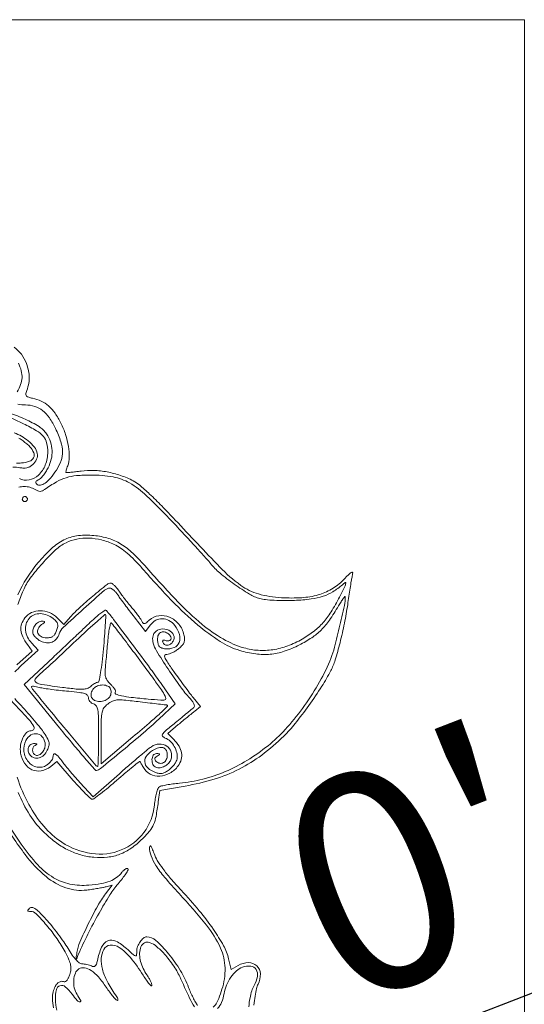
# Model space of a CAD drawing. Units: inches. Extents: x 2656 to 9931, y 1941 to 3068.
# Tile 41 of 46: x 2854 to 2868, y 2967 to 2994. Entities that reach past the tile are written whole.
import ezdxf

# ---------------------------------------------------------------- set-up
doc = ezdxf.new("R2010")
doc.units = ezdxf.units.IN
for name, color, linetype, lineweight in [('A-ANNO-DIMS', 2, 'Continuous', 18), ('A-ELEV-FNSH', 8, 'Continuous', 13), ('A-ELEV-ORN', 8, 'Continuous', 13)]:
    doc.layers.add(name, color=color, linetype=linetype, lineweight=lineweight)
doc.styles.get("Standard").update_dxf_attribs({"font": 'arial.ttf'})
doc.dimstyles.new('ISO-25', dxfattribs={"dimtxt": 6, "dimasz": 2.5, "dimexe": 1.25, "dimexo": 0.625, "dimtad": 1, "dimdec": 0, "dimlunit": 3, "dimtxsty": 'Standard', "dimcen": 2.5, "dimadec": 0, "dimazin": 0, "dimtfac": 1, "dimtdec": 0, "dimtmove": 0, "dimatfit": 3, "dimfxl": 1, "dimarcsym": 0})

# ---------------------------------------------------------------- blocks, each defined once
blk = doc.blocks.new('*D166')
at = {"layer": 'A-ANNO-DIMS', "color": 0, "lineweight": -2, "transparency": 16777216}
for p, q in [((2884.455, 2990.075), (2890.436, 2974.616)), ((2876.883, 2987.145), (2882.863, 2971.687)), ((2887.653, 2974.88), (2884.744, 2973.755)), ((2882.412, 2972.852), (2864.04, 2965.744))]:
    blk.add_line(p, q, dxfattribs=at)
at = {"layer": 'A-ANNO-DIMS', "color": 0, "transparency": 16777216}
for points in [[(2887.503, 2975.269), (2887.803, 2974.491), (2889.985, 2975.782)], [(2884.594, 2974.143), (2884.894, 2973.366), (2882.412, 2972.852)]]:
    blk.add_solid(points, dxfattribs=at)
at = {"layer": 'Defpoints', "color": 0, "transparency": 16777216}
for p in [(2884.229, 2990.658), (2876.657, 2987.728), (2882.412, 2972.852)]:
    blk.add_point(p, dxfattribs=at)
at = {"layer": 'A-ANNO-DIMS', "color": 0, "transparency": 16777216, "insert": (2870.73, 2972.287), "char_height": 6, "attachment_point": 5, "rotation": 21.1508}
blk.add_mtext('0\'-8"', dxfattribs=at)

msp = doc.modelspace()

# ---------------------------------------------------------------- linework, layer by layer
at = {"layer": 'A-ELEV-FNSH'}
msp.add_lwpolyline([(2826.64, 2994.347), (2868.226, 2994.347), (2868.226, 2892.035), (2826.64, 2892.035)], close=True, dxfattribs=at)
at = {"layer": 'A-ELEV-ORN'}
for points in [[(2854.23, 2972.992, 0.048806), (2854.547, 2972.366, 0.063105), (2854.957, 2971.872, 0.02947), (2855.295, 2971.591, 0.044031), (2855.623, 2971.392, 0.047712), (2855.96, 2971.264, 0.044288), (2856.323, 2971.198, 0.049374), (2856.702, 2971.201, 0.064618), (2857.039, 2971.282, 0.0621), (2857.354, 2971.45, 0.04132), (2857.668, 2971.712, 0.02581), (2857.866, 2971.929, 0.071696), (2857.973, 2972.105, 0.05657), (2858.04, 2972.327, 0.011722), (2858.102, 2972.73), (2858.144, 2973.048), (2858.842, 2973.168, 0.031548), (2859.647, 2973.358, 0.043232), (2860.338, 2973.635, 0.043767), (2860.964, 2974.024, 0.033519), (2861.576, 2974.549, 0.030431), (2861.884, 2974.892, 0.012266), (2862.265, 2975.395, 0.012368), (2862.625, 2975.924, 0.025654), (2862.874, 2976.357, 0.043147), (2862.994, 2976.651, 0.012156), (2863.128, 2977.129, 0.012381), (2863.251, 2977.667, 0.014486), (2863.341, 2978.184, -0.001676), (2863.374, 2978.412, -0.001753), (2863.409, 2978.637, -0.001681), (2863.44, 2978.83, -0.007763), (2863.46, 2978.942, 0.019715), (2863.479, 2979.064, 0.552387), (2863.458, 2979.081, 0.111126), (2863.41, 2979.051, 0.002476), (2863.214, 2978.857, -0.063383), (2862.893, 2978.609, -0.063935), (2862.522, 2978.45, -0.054142), (2862.07, 2978.373, -0.029361), (2861.506, 2978.372, -0.053891), (2860.87, 2978.477, -0.09017), (2860.384, 2978.713, -0.042819), (2859.805, 2979.219, -0.004549), (2858.572, 2980.52, 0.007082), (2858.2, 2980.909, 0.010597), (2857.862, 2981.237, 0.010585), (2857.58, 2981.49, 0.059203), (2857.412, 2981.603, 0.036247), (2857.06, 2981.751, 0.035563), (2856.689, 2981.848, 0.036527), (2856.318, 2981.89, 0.044145), (2855.968, 2981.872, -0.004618), (2855.815, 2981.852, -0.007219), (2855.683, 2981.839, -0.002709), (2855.57, 2981.829, -0.203128), (2855.553, 2981.835, -0.261874), (2855.548, 2981.849, -0.014563), (2855.558, 2981.896, -0.019407), (2855.574, 2981.954, -0.012699), (2855.597, 2982.02, 0.08819), (2855.641, 2982.25, 0.042084), (2855.618, 2982.552, 0.038933), (2855.539, 2982.881, 0.03792), (2855.41, 2983.197, 0.036437), (2855.247, 2983.471, 0.060016), (2855.067, 2983.671, 0.06765), (2854.863, 2983.806, 0.063263), (2854.625, 2983.886, -0.025868), (2854.519, 2983.913, -0.107249), (2854.462, 2983.945, -0.189099), (2854.44, 2983.988, -0.116621), (2854.448, 2984.044, 0.038233), (2854.511, 2984.253, 0.051641), (2854.534, 2984.449, 0.05259), (2854.515, 2984.642, 0.041783), (2854.456, 2984.844, 0.070095), (2854.315, 2985.099, 0.078135), (2854.113, 2985.294, 0.079077)], [(2854.233, 2984.857, -0.044451), (2854.313, 2984.64, -0.078218), (2854.334, 2984.45, -0.079048), (2854.296, 2984.264, -0.046304), (2854.196, 2984.059, 0.047957)], [(2854.218, 2983.718, 0.03751), (2854.433, 2983.701, -0.076239), (2854.688, 2983.661, -0.090313), (2854.903, 2983.546, -0.076144), (2855.09, 2983.345, -0.038724), (2855.261, 2983.045, -0.028856), (2855.408, 2982.681, -0.076946), (2855.456, 2982.407, -0.092728), (2855.415, 2982.161, -0.056238), (2855.283, 2981.897, -0.029077), (2855.122, 2981.678, -0.064736), (2854.971, 2981.537, -0.108333), (2854.842, 2981.481, -0.248543), (2854.744, 2981.512, -0.080101), (2854.718, 2981.548, -0.211882), (2854.716, 2981.579, -0.164265), (2854.739, 2981.606, -0.045944), (2854.79, 2981.631, 0.10487), (2854.846, 2981.668, 0.027488), (2854.918, 2981.748, 0.026679), (2854.991, 2981.85, 0.024525), (2855.055, 2981.962, 0.060506), (2855.142, 2982.199, 0.069274), (2855.164, 2982.44, 0.069972), (2855.12, 2982.676, 0.063577), (2855.012, 2982.898, 0.107608), (2854.805, 2983.101, 0.034268), (2854.424, 2983.306, 0.034451), (2853.986, 2983.469, 0.051823)], [(2853.842, 2983.44), (2854.371, 2983.182, -0.01869), (2854.737, 2982.986, -0.082984), (2854.924, 2982.831, -0.119266), (2855.015, 2982.653, -0.059157), (2855.045, 2982.4, -0.092228), (2854.978, 2982.042, -0.113061), (2854.789, 2981.761, -0.138967), (2854.528, 2981.626, -0.173005), (2854.26, 2981.665, -0.048254)], [(2854.084, 2981.976, -0.070536), (2854.276, 2981.965, 0.042314), (2854.38, 2981.954, 0.065901), (2854.469, 2981.963, 0.070033), (2854.549, 2981.994, 0.055283), (2854.625, 2982.049, 0.102685), (2854.735, 2982.2, 0.153719), (2854.755, 2982.361, 0.121971), (2854.677, 2982.531, 0.052991), (2854.502, 2982.71, 0.090302), (2854.115, 2982.926, 0.071489)], [(2854.25, 2982.779, -0.019972), (2854.361, 2982.707, -0.019921), (2854.467, 2982.624, -0.031903), (2854.55, 2982.545, -0.083683), (2854.659, 2982.379, -0.226186), (2854.654, 2982.241, -0.19243), (2854.54, 2982.143, -0.0618), (2854.317, 2982.096, -0.017844), (2854.177, 2982.089, -0.111032)], [(2854.248, 2981.426, -0.071275), (2854.394, 2981.446, -0.065833), (2854.553, 2981.424, -0.072585), (2854.695, 2981.362, 0.038782), (2854.771, 2981.322, 0.100434), (2854.831, 2981.31, 0.107028), (2854.889, 2981.322, 0.047721), (2854.957, 2981.361, -0.022709), (2855.289, 2981.574, -0.055018), (2855.556, 2981.69, -0.05461), (2855.842, 2981.747, -0.022094), (2856.241, 2981.763, -0.042989), (2856.854, 2981.709, -0.087275), (2857.308, 2981.544, -0.060467), (2857.777, 2981.192, -0.012478), (2858.505, 2980.458, -0.001643), (2858.857, 2980.083, -0.002101), (2859.179, 2979.734, -0.001624), (2859.446, 2979.44, -0.017799), (2859.549, 2979.318, 0.052744), (2859.8, 2979.059, 0.019241), (2860.205, 2978.746, 0.018442), (2860.624, 2978.47, 0.070736), (2860.911, 2978.347, 0.041481), (2861.066, 2978.319, 0.011613), (2861.311, 2978.301, 0.01162), (2861.59, 2978.293, 0.011922), (2861.867, 2978.298, 0.019879), (2862.329, 2978.337, 0.048301), (2862.662, 2978.411, 0.059001), (2862.933, 2978.537, 0.045481), (2863.194, 2978.732, -0.048141), (2863.271, 2978.789, -0.666317), (2863.291, 2978.774, -0.055029), (2863.257, 2978.682, -0.002672), (2863.111, 2978.39, -0.020952), (2862.881, 2977.98, -0.042924), (2862.661, 2977.684, -0.047406), (2862.409, 2977.449, -0.031918), (2862.083, 2977.229, -0.04403), (2861.682, 2977.041, -0.050837), (2861.274, 2976.936, -0.052866), (2860.867, 2976.918, -0.055097), (2860.471, 2976.987, -0.060568), (2859.896, 2977.232, -0.041968), (2859.315, 2977.636, -0.029176), (2858.636, 2978.269, -0.010066), (2857.729, 2979.258, 0.026051), (2857.356, 2979.64, 0.056179), (2857.026, 2979.882, 0.064448), (2856.68, 2980.025, 0.045684), (2856.266, 2980.096, 0.056703), (2855.845, 2980.082, 0.081774), (2855.491, 2979.969, 0.069441), (2855.151, 2979.731, 0.030248), (2854.772, 2979.332, 0.06803), (2854.218, 2978.456, 0.054859)], [(2854.219, 2978.186, -0.013623), (2854.371, 2978.577, -0.060131), (2854.56, 2978.909, -0.023236), (2854.896, 2979.32, -0.022829), (2855.263, 2979.693, -0.071671), (2855.551, 2979.893, -0.067619), (2855.85, 2979.994, -0.057199), (2856.182, 2980.02, -0.053478), (2856.533, 2979.969, -0.045502), (2856.886, 2979.844, -0.043482), (2857.057, 2979.746, -0.025451), (2857.244, 2979.602, -0.021958), (2857.445, 2979.414, -0.014566), (2857.66, 2979.182, 0.012962), (2858.488, 2978.28, 0.025737), (2859.197, 2977.618, 0.032645), (2859.815, 2977.164, 0.068696), (2860.355, 2976.915, 0.039649), (2860.796, 2976.819, 0.056839), (2861.196, 2976.81, 0.056725), (2861.588, 2976.891, 0.039291), (2862.005, 2977.066, 0.028741), (2862.348, 2977.268, 0.048454), (2862.605, 2977.479, 0.04403), (2862.833, 2977.75, 0.019532), (2863.086, 2978.144, -0.007841), (2863.158, 2978.261, -0.016312), (2863.218, 2978.35, -0.02101), (2863.262, 2978.405, -0.690309), (2863.273, 2978.401, -0.056809), (2863.248, 2978.157, -0.004737), (2863.106, 2977.537, -0.005838), (2862.953, 2976.926, -0.03674), (2862.848, 2976.622, -0.030818), (2862.518, 2975.966, -0.025736), (2862.09, 2975.312, -0.026372), (2861.614, 2974.729, -0.040546), (2861.139, 2974.283, -0.0314), (2860.555, 2973.876, -0.036475), (2859.954, 2973.567, -0.037744), (2859.332, 2973.358, -0.038614), (2858.691, 2973.246, 0.009153), (2858.505, 2973.225, 0.011505), (2858.334, 2973.198, 0.009742), (2858.192, 2973.17, 0.084331), (2858.133, 2973.145, 0.168872), (2858.095, 2973.099, 0.021132), (2858.055, 2972.974, 0.02295), (2858.02, 2972.815, 0.017154), (2857.996, 2972.638, -0.133176), (2857.706, 2971.885, -0.140208), (2857.079, 2971.4, -0.131546), (2856.258, 2971.301, -0.111133), (2855.437, 2971.614, -0.069431), (2854.936, 2972.056, -0.052987), (2854.521, 2972.659, -0.047105), (2854.202, 2973.409, -0.034503)], [(2853.854, 2975.717), (2854.274, 2975.276, -0.008047), (2854.548, 2974.977, -0.057105), (2854.661, 2974.817, -0.266162), (2854.66, 2974.737, -0.263313), (2854.589, 2974.697, 0.195413), (2854.462, 2974.646, 0.088723), (2854.356, 2974.497, 0.075041), (2854.294, 2974.293, 0.076162), (2854.295, 2974.08, 0.102944), (2854.404, 2973.795, 0.145746), (2854.609, 2973.618, 0.154529), (2854.867, 2973.588, 0.119579), (2855.127, 2973.706), (2855.298, 2973.841), (2855.752, 2973.322, 0.00697), (2855.931, 2973.123, 0.010456), (2856.093, 2972.955, 0.005693), (2856.233, 2972.819, 0.183501), (2856.276, 2972.801, 0.171151), (2856.322, 2972.815, 0.003919), (2856.507, 2972.956, 0.008308), (2856.723, 2973.129, 0.005478), (2856.964, 2973.335, -0.003428), (2857.202, 2973.539, -0.005779), (2857.405, 2973.706, -0.001369), (2857.582, 2973.848, -0.462514), (2857.597, 2973.845, -0.001255), (2857.607, 2973.828, -0.000112), (2857.631, 2973.784, -0.000146), (2857.659, 2973.733, -0.000114), (2857.69, 2973.677, 0.151544), (2857.875, 2973.499, 0.129065), (2858.141, 2973.443, 0.115479), (2858.424, 2973.524, 0.10603), (2858.652, 2973.724, 0.093022), (2858.737, 2973.898, 0.109096), (2858.746, 2974.081, 0.096382), (2858.676, 2974.269, 0.058894), (2858.529, 2974.455), (2858.362, 2974.622), (2858.655, 2974.865, -0.000702), (2858.779, 2974.967, -0.000611), (2858.91, 2975.074, -0.000614), (2859.028, 2975.171, -0.001815), (2859.109, 2975.236), (2859.269, 2975.365), (2859.069, 2975.612, -0.008149), (2858.97, 2975.738, -0.002788), (2858.829, 2975.925, -0.002771), (2858.676, 2976.133, -0.003198), (2858.533, 2976.332, -0.004981), (2858.344, 2976.606, -0.052517), (2858.28, 2976.725, -0.263875), (2858.288, 2976.781, -0.235291), (2858.341, 2976.807, 0.081921), (2858.409, 2976.818, 0.031994), (2858.497, 2976.855, 0.030613), (2858.589, 2976.907, 0.033279), (2858.672, 2976.969, 0.031381), (2858.768, 2977.063, 0.094797), (2858.816, 2977.141, 0.102826), (2858.829, 2977.228, 0.04083), (2858.813, 2977.347, 0.117062), (2858.671, 2977.641, 0.122846), (2858.415, 2977.834, 0.133996), (2858.115, 2977.874, 0.15172), (2857.854, 2977.752, -0.012802), (2857.76, 2977.672, -0.163935), (2857.717, 2977.656, -0.247353), (2857.682, 2977.673, -0.031273), (2857.636, 2977.745, 0.02546), (2857.596, 2977.808, 0.007786), (2857.53, 2977.9, 0.007771), (2857.452, 2978, 0.008425), (2857.373, 2978.095, -0.007622), (2857.288, 2978.197, -0.004686), (2857.191, 2978.321, -0.004697), (2857.097, 2978.444, -0.008369), (2857.023, 2978.548, 0.020166), (2856.957, 2978.635, 0.026507), (2856.889, 2978.709, 0.025902), (2856.828, 2978.763, 0.170141), (2856.791, 2978.777, 0.171394), (2856.685, 2978.739, 0.004434), (2856.29, 2978.415, 0.010022), (2855.914, 2978.087, 0.029145), (2855.673, 2977.841), (2855.491, 2977.633), (2855.306, 2977.818, 0.097051), (2855.091, 2977.963, 0.101521), (2854.84, 2978.013, 0.106808), (2854.599, 2977.96, 0.118645), (2854.413, 2977.812, 0.083046), (2854.323, 2977.648, 0.107638), (2854.303, 2977.478, 0.089753), (2854.355, 2977.292, 0.043112), (2854.482, 2977.078), (2854.616, 2976.893), (2854.189, 2976.521, -0.002591)], [(2854.134, 2976.325, -0.010744), (2854.313, 2976.495), (2854.781, 2976.921), (2854.597, 2977.121, -0.155547), (2854.432, 2977.472, -0.216304), (2854.532, 2977.8, -0.225193), (2854.839, 2977.932, -0.162288), (2855.194, 2977.799, -0.034107), (2855.28, 2977.719, -0.120439), (2855.317, 2977.654, -0.11998), (2855.32, 2977.579, -0.033726), (2855.288, 2977.465, -0.042669), (2855.243, 2977.364, -0.109987), (2855.19, 2977.305, -0.11168), (2855.117, 2977.274, -0.044776), (2855.009, 2977.264, -0.113648), (2854.859, 2977.299, -0.193773), (2854.774, 2977.393, -0.203175), (2854.78, 2977.515, -0.123162), (2854.875, 2977.629, 0.009914), (2854.943, 2977.681, 0.18349), (2854.957, 2977.704, 0.430874), (2854.947, 2977.718, 0.029344), (2854.891, 2977.722, 0.131977), (2854.787, 2977.694, 0.097096), (2854.696, 2977.614, 0.09479), (2854.641, 2977.505, 0.11829), (2854.636, 2977.391, 0.102909), (2854.659, 2977.337, 0.045051), (2854.709, 2977.276, 0.042034), (2854.776, 2977.218, 0.043851), (2854.851, 2977.174, 0.086985), (2855.014, 2977.128, 0.117271), (2855.164, 2977.148, 0.12305), (2855.285, 2977.233, 0.102014), (2855.362, 2977.37, -0.128126), (2855.475, 2977.55, -0.005371), (2856.036, 2978.065, -0.004251), (2856.617, 2978.579, -0.180742), (2856.77, 2978.636, -0.144837), (2856.813, 2978.623, -0.037592), (2856.872, 2978.578, -0.035008), (2856.933, 2978.515, -0.029536), (2856.99, 2978.44, 0.010586), (2857.061, 2978.339, 0.003006), (2857.175, 2978.184, 0.003027), (2857.306, 2978.011, 0.0032), (2857.436, 2977.843), (2857.753, 2977.44), (2857.882, 2977.616, -0.108504), (2858.032, 2977.748, -0.130694), (2858.213, 2977.793, -0.126191), (2858.398, 2977.743, -0.097356), (2858.557, 2977.607, -0.091159), (2858.687, 2977.359, -0.171125), (2858.679, 2977.136, -0.203504), (2858.538, 2976.993, -0.127397), (2858.302, 2976.96, -0.044798), (2858.202, 2976.981, -0.12164), (2858.14, 2977.018, -0.123492), (2858.103, 2977.079, -0.046878), (2858.082, 2977.177, -0.101051), (2858.094, 2977.317, -0.181101), (2858.163, 2977.408, -0.19807), (2858.269, 2977.427, -0.119669), (2858.386, 2977.37, -0.107943), (2858.446, 2977.293, -0.223895), (2858.446, 2977.22, -0.255959), (2858.391, 2977.179, -0.126114), (2858.303, 2977.189, 0.052946), (2858.261, 2977.2, 0.18302), (2858.234, 2977.195, 0.245328), (2858.223, 2977.175, 0.090495), (2858.228, 2977.141, 0.165813), (2858.277, 2977.077, 0.175052), (2858.354, 2977.057, 0.135976), (2858.442, 2977.091, 0.091769), (2858.515, 2977.171, 0.251134), (2858.527, 2977.338, 0.182135), (2858.392, 2977.474, 0.145113), (2858.175, 2977.505, 0.184648), (2858, 2977.406, 0.084785), (2857.968, 2977.351, 0.05344), (2857.95, 2977.279, 0.049465), (2857.947, 2977.199, 0.047296), (2857.959, 2977.118, 0.078783), (2858.05, 2976.905, 0.006742), (2858.374, 2976.404, 0.009495), (2858.717, 2975.91, 0.029074), (2858.974, 2975.593, -0.027455), (2859.042, 2975.51, -0.054375), (2859.085, 2975.437, -0.079921), (2859.1, 2975.378, -0.239417), (2859.085, 2975.341, -0.008268), (2859.04, 2975.302, -0.000536), (2858.908, 2975.192, -0.000781), (2858.75, 2975.062, -0.000582), (2858.575, 2974.919, 0.004086), (2858.296, 2974.687, 0.071765), (2858.218, 2974.599, 0.344701), (2858.223, 2974.543, 0.115993), (2858.296, 2974.494, -0.101431), (2858.433, 2974.407, -0.071341), (2858.545, 2974.262, -0.07075), (2858.613, 2974.09, -0.095835), (2858.621, 2973.923, -0.080311), (2858.598, 2973.851, -0.037754), (2858.547, 2973.767, -0.036154), (2858.479, 2973.685, -0.042211), (2858.404, 2973.618, -0.031154), (2858.298, 2973.549, -0.078619), (2858.212, 2973.517, -0.088551), (2858.126, 2973.515, -0.04758), (2858.024, 2973.541, -0.097769), (2857.81, 2973.668, -0.202366), (2857.728, 2973.842, -0.195982), (2857.795, 2974.025, -0.092111), (2857.998, 2974.181, -0.066337), (2858.144, 2974.232, -0.160123), (2858.255, 2974.219, -0.189863), (2858.326, 2974.146, -0.097673), (2858.351, 2974.019, -0.11267), (2858.323, 2973.897, -0.15229), (2858.246, 2973.814, -0.175637), (2858.144, 2973.796, -0.153038), (2858.048, 2973.847, -0.054276), (2858.013, 2973.89, -0.181249), (2858.005, 2973.926, -0.169745), (2858.022, 2973.959, -0.04647), (2858.07, 2973.996, 0.011499), (2858.128, 2974.034, 0.316019), (2858.133, 2974.05, 0.323507), (2858.12, 2974.061, 0.0118), (2858.052, 2974.063, 0.256259), (2857.965, 2974.017, 0.136609), (2857.928, 2973.897, 0.118941), (2857.955, 2973.763, 0.193325), (2858.039, 2973.685, 0.128884), (2858.15, 2973.673, 0.082462), (2858.274, 2973.713, 0.079442), (2858.383, 2973.793, 0.103336), (2858.45, 2973.896, 0.162282), (2858.459, 2974.107, 0.178644), (2858.339, 2974.272, 0.162217), (2858.13, 2974.328, 0.135168), (2857.911, 2974.254, 0.024279), (2857.814, 2974.182, 0.002281), (2857.586, 2973.991, 0.002921), (2857.316, 2973.761, 0.002293), (2857.026, 2973.509), (2856.299, 2972.87), (2855.936, 2973.266, -0.005143), (2855.786, 2973.432, -0.004892), (2855.638, 2973.605, -0.004859), (2855.51, 2973.759, -0.017251), (2855.432, 2973.862, 0.022274), (2855.326, 2973.999, 0.122686), (2855.25, 2974.053, 0.382658), (2855.205, 2974.037, 0.122775), (2855.186, 2973.96, -0.123438), (2855.174, 2973.912, -0.045037), (2855.135, 2973.854, -0.041261), (2855.079, 2973.794, -0.038647), (2855.014, 2973.744, -0.195849), (2854.751, 2973.692, -0.172068), (2854.509, 2973.835, -0.146822), (2854.386, 2974.122, -0.14475), (2854.441, 2974.43, -0.145358), (2854.581, 2974.579, -0.18994), (2854.764, 2974.608, -0.192587), (2854.916, 2974.504, -0.148544), (2854.975, 2974.31, -0.099823), (2854.949, 2974.184, -0.09492), (2854.877, 2974.076, -0.118377), (2854.783, 2974.017, -0.22271), (2854.696, 2974.027, -0.143286), (2854.642, 2974.087, -0.125973), (2854.626, 2974.17, -0.129659), (2854.651, 2974.249, -0.155794), (2854.711, 2974.299, 0.05712), (2854.738, 2974.314, 0.451941), (2854.739, 2974.326, 0.17712), (2854.72, 2974.336, 0.021621), (2854.674, 2974.34, 0.151335), (2854.574, 2974.314, 0.166009), (2854.511, 2974.237, 0.147761), (2854.504, 2974.129, 0.116066), (2854.556, 2974.025, 0.143279), (2854.669, 2973.949, 0.145863), (2854.804, 2973.946, 0.124212), (2854.934, 2974.021, 0.090292), (2855.033, 2974.157, 0.040581), (2855.079, 2974.278, 0.11715), (2855.084, 2974.367, 0.085281), (2855.048, 2974.465, 0.015338), (2854.945, 2974.631, 0.021888), (2854.845, 2974.769, 0.006806), (2854.682, 2974.968, 0.00679), (2854.494, 2975.185, 0.007434), (2854.306, 2975.391, -0.009083), (2854.131, 2975.583, -0.012896)], [(2853.752, 2972.257, 0.021715), (2854.422, 2971.271, 0.060142), (2854.998, 2970.664, 0.08968), (2855.55, 2970.354, 0.114067), (2856.129, 2970.293, 0.006163), (2856.279, 2970.313, 0.005657), (2856.432, 2970.338, 0.00566), (2856.568, 2970.362, 0.01848), (2856.657, 2970.383), (2856.828, 2970.43), (2856.644, 2970.188, 0.036444), (2856.428, 2969.858, 0.012767), (2856.166, 2969.356, 0.011276), (2855.934, 2968.852, 0.063974), (2855.852, 2968.569, 0.001451), (2855.828, 2968.414, 0.181535), (2855.833, 2968.395, 0.596344), (2855.842, 2968.396, 0.002901), (2855.891, 2968.508, -0.013568), (2856.157, 2969.077, -0.011969), (2856.464, 2969.656, -0.011894), (2856.763, 2970.161, -0.039983), (2856.992, 2970.469, 0.013147), (2857.111, 2970.613, 0.021325), (2857.204, 2970.742, 0.016747), (2857.269, 2970.848, 0.336738), (2857.264, 2970.884, 0.261988), (2857.237, 2970.891, 0.07607), (2857.195, 2970.874, 0.055128), (2857.146, 2970.837, 0.034076), (2857.097, 2970.783, -0.064471), (2856.947, 2970.637, -0.068156), (2856.767, 2970.537, -0.051658), (2856.527, 2970.471, -0.020091), (2856.184, 2970.429, -0.069802), (2855.66, 2970.459, -0.087335), (2855.205, 2970.635, -0.071196), (2854.773, 2970.988, -0.03148), (2854.308, 2971.564, -0.028331), (2853.89, 2972.23, -0.037211)], [(2860.744, 2967.112, -0.013655), (2860.78, 2967.361, -0.013252), (2860.821, 2967.572, -0.061857), (2860.863, 2967.689, 0.124401), (2860.927, 2967.975, 0.199008), (2860.826, 2968.2, 0.198758), (2860.596, 2968.289, 0.124145), (2860.313, 2968.209), (2860.122, 2968.1), (2860.048, 2968.395, 0.064485), (2859.907, 2968.753, 0.025357), (2859.626, 2969.206, 0.021822), (2859.234, 2969.722, 0.014076), (2858.738, 2970.287, -0.009089), (2858.443, 2970.616, -0.018684), (2858.227, 2970.885, -0.023762), (2858.075, 2971.111, -0.049716), (2857.984, 2971.303, 0.009579), (2857.931, 2971.442, 0.057989), (2857.894, 2971.51, 0.494324), (2857.874, 2971.51, 0.169739), (2857.861, 2971.477, 0.094064), (2857.902, 2971.239, 0.052611), (2858.034, 2970.974, 0.034572), (2858.276, 2970.647, 0.011168), (2858.678, 2970.196, -0.017859), (2859.437, 2969.32, -0.064429), (2859.822, 2968.691, -0.098957), (2859.948, 2968.14, -0.085056), (2859.863, 2967.55, -0.012244), (2859.773, 2967.294, -0.050047), (2859.7, 2967.146, -0.082559), (2859.62, 2967.056, -0.084337)], [(2859.191, 2967.103, -0.033217), (2859.132, 2967.192, -0.013391), (2859.063, 2967.321, -0.013182), (2858.995, 2967.464, -0.01629), (2858.94, 2967.601, 0.049726), (2858.718, 2968.064, 0.035908), (2858.385, 2968.531, 0.033641), (2858.033, 2968.902, 0.188442), (2857.783, 2969, 0.179522), (2857.693, 2968.967, 0.064192), (2857.601, 2968.864, 0.060737), (2857.53, 2968.73, 0.090549), (2857.507, 2968.6, -0.034213), (2857.5, 2968.495, -0.454167), (2857.471, 2968.476, -0.112875), (2857.415, 2968.506, -0.003465), (2857.22, 2968.68, 0.065906), (2856.931, 2968.879, 0.220463), (2856.706, 2968.887, 0.194034), (2856.535, 2968.718, 0.051181), (2856.417, 2968.343, -0.02807), (2856.391, 2968.245, -0.128317), (2856.359, 2968.196, -0.202844), (2856.316, 2968.18, -0.086807), (2856.255, 2968.194, 0.028592), (2856.199, 2968.214, 0.016152), (2856.129, 2968.233, 0.016083), (2856.057, 2968.247, 0.025339), (2855.995, 2968.253, -0.14779), (2855.918, 2968.281, -0.045711), (2855.827, 2968.364, -0.0349), (2855.723, 2968.494, -0.016518), (2855.608, 2968.674, 0.017394), (2855.487, 2968.86, 0.009411), (2855.327, 2969.082, 0.009364), (2855.156, 2969.301, 0.014576), (2854.999, 2969.483, 0.008739), (2854.805, 2969.687, 0.049377), (2854.689, 2969.784, 0.121836), (2854.609, 2969.813, 0.224101), (2854.545, 2969.791, 0.019744), (2854.5, 2969.744, 0.250542), (2854.494, 2969.721, 0.310357), (2854.511, 2969.707, 0.026874), (2854.568, 2969.703, -0.201397), (2854.721, 2969.639, -0.017461), (2855.013, 2969.32, -0.023476), (2855.304, 2968.944, -0.033254), (2855.524, 2968.582, -0.012956), (2855.632, 2968.36, -0.054577), (2855.679, 2968.219, -0.078868), (2855.685, 2968.099, -0.047866), (2855.656, 2967.959, -0.033647), (2855.623, 2967.871, -0.056383), (2855.582, 2967.804, -0.078505), (2855.54, 2967.764, -0.2466), (2855.502, 2967.759, 0.143304), (2855.409, 2967.767, 0.134185), (2855.323, 2967.724, 0.094582), (2855.25, 2967.627, 0.044481), (2855.193, 2967.479, 0.086203), (2855.174, 2967.3, 0.028596), (2855.206, 2967.037, 0.019917)], [(2855.3, 2966.971, -0.074704), (2855.256, 2967.264, -0.0517), (2855.285, 2967.54, -0.268106), (2855.383, 2967.649, -0.26418), (2855.528, 2967.62, -0.050662), (2855.719, 2967.416, 0.014757), (2855.862, 2967.24, 0.200757), (2855.934, 2967.204, 0.591687), (2855.956, 2967.238, 0.020346), (2855.855, 2967.406, -0.092945), (2855.779, 2967.588, -0.070995), (2855.765, 2967.803, -0.076437), (2855.809, 2967.996, -0.159371), (2855.907, 2968.114, -0.188565), (2856.061, 2968.143, -0.101102), (2856.242, 2968.069, -0.066365), (2856.445, 2967.89, -0.030329), (2856.66, 2967.61, 0.010594), (2856.76, 2967.47, 0.015621), (2856.854, 2967.351, 0.010823), (2856.936, 2967.258, 0.206582), (2856.97, 2967.242, 0.394853), (2856.984, 2967.255, 0.100672), (2856.98, 2967.288, 0.051468), (2856.957, 2967.339, 0.023996), (2856.918, 2967.4, -0.034033), (2856.688, 2967.77, -0.058983), (2856.557, 2968.107, -0.074397), (2856.526, 2968.403, -0.112085), (2856.595, 2968.653, -0.256109), (2856.775, 2968.77, -0.165608), (2857.022, 2968.707, -0.077829), (2857.333, 2968.426, -0.028236), (2857.681, 2967.942, 0.010809), (2857.775, 2967.801, 0.023826), (2857.854, 2967.699, 0.04175), (2857.908, 2967.644, 0.630406), (2857.927, 2967.653, 0.091265), (2857.919, 2967.702, 0.023548), (2857.888, 2967.776, 0.023164), (2857.845, 2967.858, 0.021735), (2857.793, 2967.938, -0.043249), (2857.683, 2968.125, -0.050103), (2857.613, 2968.318, -0.053978), (2857.587, 2968.508, -0.069071), (2857.606, 2968.684, -0.159155), (2857.69, 2968.818, -0.22727), (2857.825, 2968.852, -0.116696), (2858.012, 2968.765, -0.035451), (2858.246, 2968.554, -0.024342), (2858.369, 2968.411, -0.01586), (2858.498, 2968.236, -0.015959), (2858.614, 2968.057, -0.029113), (2858.694, 2967.903, 0.004022), (2858.97, 2967.304, 0.041294), (2859.105, 2967.067, 0.109032)], [(2859.739, 2967.018, 0.102309), (2859.854, 2967.189, 0.057096), (2859.922, 2967.431, -0.058464), (2859.988, 2967.665, -0.055388), (2860.107, 2967.882, -0.058702), (2860.262, 2968.056, -0.090107), (2860.434, 2968.159, -0.114465), (2860.66, 2968.19, -0.233443), (2860.809, 2968.099, -0.190961), (2860.845, 2967.905, -0.081887), (2860.752, 2967.654, 0.053801), (2860.686, 2967.504, 0.032), (2860.639, 2967.314, 0.023375), (2860.606, 2967.062, 0.009261)]]:
    msp.add_lwpolyline(points, format="xyb", dxfattribs=at)
for points in [[(2854.342, 2981.098, 0.099038), (2854.347, 2981.071, 0.097945), (2854.362, 2981.048, 0.097945), (2854.385, 2981.033, 0.099038), (2854.412, 2981.027, 0.099038), (2854.439, 2981.033, 0.097945), (2854.462, 2981.048, 0.097945), (2854.477, 2981.071, 0.099038), (2854.482, 2981.098, 0.099038), (2854.477, 2981.124, 0.097945), (2854.462, 2981.147, 0.097945), (2854.439, 2981.163, 0.099038), (2854.412, 2981.168, 0.099038), (2854.385, 2981.163, 0.097945), (2854.362, 2981.147, 0.097945), (2854.347, 2981.124, 0.099038)], [(2856.308, 2977.773, -0.000343), (2856.136, 2977.611, -0.000082), (2855.851, 2977.342, -0.000084), (2855.523, 2977.034, -0.000084), (2855.194, 2976.724), (2854.396, 2975.973), (2855.371, 2974.777, 0.002756), (2855.748, 2974.32, 0.004502), (2856.074, 2973.937, 0.000895), (2856.363, 2973.604, 0.284345), (2856.395, 2973.594, 0.108063), (2856.5, 2973.648, 0.001242), (2857.11, 2974.148, 0.004303), (2857.691, 2974.636, 0.010058), (2858.115, 2975.014), (2858.571, 2975.436), (2858.197, 2975.974, 0.00705), (2857.891, 2976.401, 0.001783), (2857.383, 2977.087, 0.00124), (2856.866, 2977.774, 0.016647), (2856.667, 2978.019, 0.356672), (2856.634, 2978.025, 0.021696), (2856.543, 2977.968, 0.0245), (2856.432, 2977.884, 0.014798)], [(2856.585, 2976.956, -0.006819), (2856.547, 2976.593, -0.012306), (2856.504, 2976.298, -0.00627), (2856.461, 2976.06, -0.358842), (2856.429, 2976.034, 0.101634), (2856.393, 2976.026, 0.028775), (2856.342, 2976.001, 0.027725), (2856.286, 2975.964, 0.026126), (2856.233, 2975.921, -0.099703), (2856.139, 2975.865, -0.075763), (2856.02, 2975.843, -0.035581), (2855.831, 2975.849, -0.005331), (2855.454, 2975.894, -0.005307), (2854.883, 2975.973, -0.10397), (2854.718, 2976.035, -0.434714), (2854.701, 2976.124, -0.059736), (2854.845, 2976.278, 0.009928), (2854.98, 2976.396, 0.001613), (2855.237, 2976.632, 0.001778), (2855.537, 2976.91, 0.001564), (2855.848, 2977.204, -0.00331), (2856.145, 2977.481, -0.005508), (2856.399, 2977.71, -0.001218), (2856.622, 2977.906, -0.394732), (2856.643, 2977.905, -0.213602), (2856.652, 2977.881, -0.001128), (2856.637, 2977.616, -0.004654), (2856.616, 2977.312, -0.002902)], [(2857.307, 2977.026, -0.001875), (2857.688, 2976.517, -0.004089), (2857.976, 2976.123, -0.004612), (2858.187, 2975.824, -0.024198), (2858.293, 2975.654, -0.131343), (2858.31, 2975.583, -0.359389), (2858.279, 2975.546, -0.063288), (2858.169, 2975.541, -0.003425), (2857.821, 2975.57, -0.005452), (2857.356, 2975.617, -0.02377), (2857.083, 2975.661, -0.043762), (2856.932, 2975.707, -0.465353), (2856.914, 2975.76, 0.229555), (2856.917, 2975.795, 0.047914), (2856.891, 2975.85, 0.041286), (2856.844, 2975.915, 0.028685), (2856.782, 2975.98, -0.04297), (2856.705, 2976.065, -0.065601), (2856.656, 2976.151, -0.06839), (2856.633, 2976.244, -0.05158), (2856.632, 2976.35, 0.000694), (2856.642, 2976.467, 0.00015), (2856.661, 2976.67, 0.000156), (2856.682, 2976.906, 0.000149), (2856.703, 2977.145, -0.009316), (2856.726, 2977.365, -0.017721), (2856.755, 2977.54, -0.016497), (2856.784, 2977.666, -0.585791), (2856.808, 2977.672, -0.024699), (2856.844, 2977.631, -0.000832), (2856.976, 2977.459, -0.001572), (2857.132, 2977.256, -0.001095)], [(2855.625, 2975.785, -0.007244), (2855.925, 2975.753, -0.048733), (2856.071, 2975.721, -0.124854), (2856.143, 2975.676, -0.192417), (2856.17, 2975.608, 0.100077), (2856.181, 2975.556, 0.071536), (2856.212, 2975.505, 0.068541), (2856.257, 2975.462, 0.076421), (2856.311, 2975.436, -0.17165), (2856.389, 2975.377, -0.106822), (2856.43, 2975.27, -0.03601), (2856.448, 2975.061, -0.00346), (2856.452, 2974.552, -0.003589), (2856.449, 2974.23, -0.005981), (2856.442, 2973.959, -0.001434), (2856.433, 2973.725, -0.401379), (2856.42, 2973.712, -0.221401), (2856.388, 2973.727, -0.000106), (2855.646, 2974.61, -0.001485), (2854.993, 2975.392, -0.007576), (2854.637, 2975.833, -0.037967), (2854.595, 2975.898, -0.471119), (2854.604, 2975.922, -0.128372), (2854.652, 2975.925, -0.005852), (2854.813, 2975.892, 0.01575), (2854.952, 2975.866, 0.00491), (2855.162, 2975.836, 0.004902), (2855.397, 2975.808, 0.005391)], [(2856.782, 2975.848, -0.134497), (2856.794, 2975.723, -0.139371), (2856.74, 2975.611, -0.122243), (2856.629, 2975.533, -0.090736), (2856.48, 2975.506, -0.106505), (2856.342, 2975.536, -0.178943), (2856.258, 2975.618, -0.17873), (2856.248, 2975.735, -0.106242), (2856.314, 2975.861, -0.135188), (2856.422, 2975.936, -0.092319), (2856.57, 2975.96, -0.100563), (2856.706, 2975.928, -0.196427)], [(2858.337, 2975.406, -0.575653), (2858.348, 2975.368, -0.013816), (2858.19, 2975.212, -0.011018), (2857.916, 2974.965, -0.002036), (2857.399, 2974.523), (2856.522, 2973.781), (2856.522, 2974.536, -0.004346), (2856.526, 2975.011, -0.045386), (2856.547, 2975.205, -0.105873), (2856.599, 2975.325, -0.069345), (2856.703, 2975.434, -0.06081), (2856.832, 2975.513, -0.090883), (2856.96, 2975.546, -0.041588), (2857.153, 2975.543, -0.004412), (2857.6, 2975.495, -0.000366), (2857.876, 2975.462, -0.000582), (2858.112, 2975.434, -0.000108), (2858.32, 2975.409, -0.030491)]]:
    msp.add_lwpolyline(points, format="xyb", close=True, dxfattribs=at)

# ---------------------------------------------------------------- dimensions: what is measured, and where the dimension line sits
at = {"layer": 'A-ANNO-DIMS'}
dim = msp.add_linear_dim(base=(2882.412, 2972.852), p1=(2884.229, 2990.658), p2=(2876.657, 2987.728), angle=201.1508, dimstyle='ISO-25', override={"dimdec": 1, "dimlfac": 1, "dimrnd": 0, "dimzin": 1, "dimdsep": 46, "dimlunit": 4, "dimfrac": 2}, dxfattribs=at)
dim.commit()
dim.dimension.update_dxf_attribs({"geometry": '*D166', "text_midpoint": (2870.73, 2972.287)})

doc.saveas('drawing.dxf')
